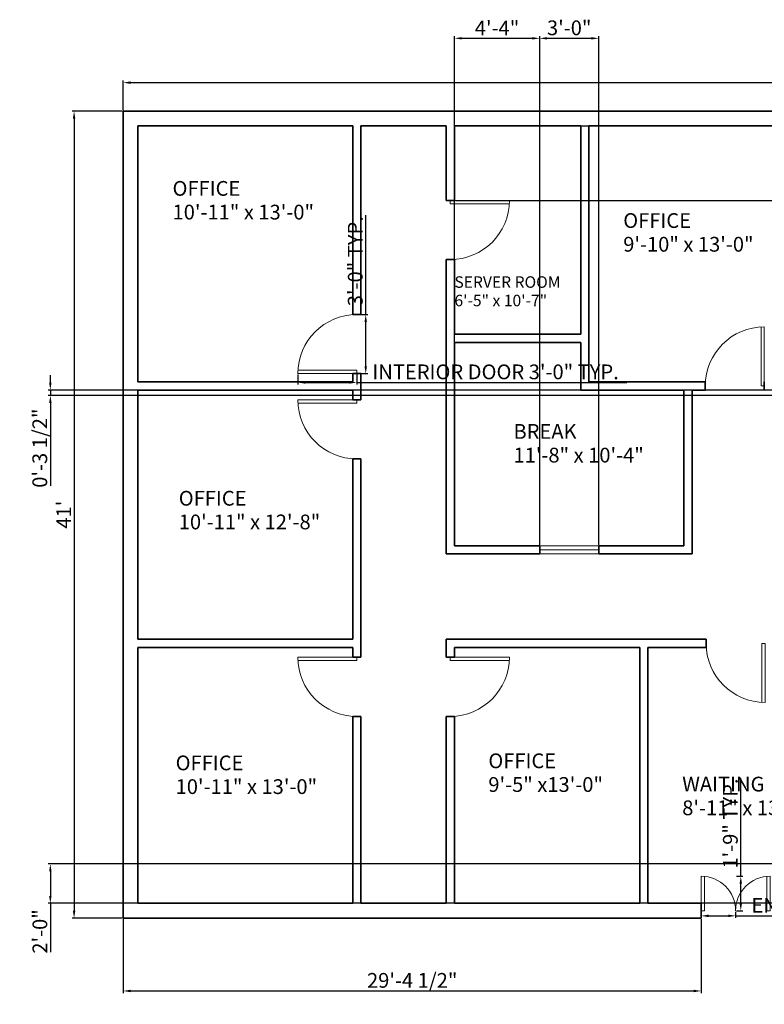
# Model space of a CAD drawing. Units: inches. Extents: x 2070 to 3026, y 1437 to 2044.
# Tile 1 of 2: x 2070 to 2524, y 1437 to 2037. Entities that reach past the tile are written whole.
import ezdxf

# ---------------------------------------------------------------- set-up
doc = ezdxf.new("R2010")
doc.units = ezdxf.units.IN
doc.layers.add('A-ANNO-DIMS', color=11, linetype='Continuous', lineweight=18, true_color=0xf27172)
doc.layers.add('A-GLAZ', color=11, linetype='Continuous', lineweight=18, true_color=0xf27172)
for name, color, linetype, lineweight in [('A-AREA-IDEN', 7, 'Continuous', 18), ('A-DOOR', 4, 'Continuous', 18), ('A-WALL', 7, 'Continuous', 35)]:
    doc.layers.add(name, color=color, linetype=linetype, lineweight=lineweight)
doc.styles.get("Standard").update_dxf_attribs({"font": 'arial.ttf'})
doc.dimstyles.new('ISO-25', dxfattribs={"dimtxt": 9, "dimasz": 4.5, "dimexe": 1.25, "dimexo": 0.625, "dimtad": 1, "dimdec": 0, "dimlunit": 3, "dimtxsty": 'Standard', "dimcen": 2.5, "dimadec": 0, "dimazin": 0, "dimtfac": 1, "dimtdec": 0, "dimtmove": 0, "dimatfit": 3, "dimfxl": 1, "dimarcsym": 0})

# ---------------------------------------------------------------- blocks, each defined once
blk = doc.blocks.new('*D3')
at = {"layer": 'A-ANNO-DIMS', "color": 0, "lineweight": -2, "transparency": 16777216}
for p, q in [((2133.31, 1981.8), (2133.31, 1999.85)), ((2973.31, 1981.8), (2973.31, 1999.85)), ((2137.81, 1998.6), (2968.81, 1998.6))]:
    blk.add_line(p, q, dxfattribs=at)
at = {"layer": 'A-ANNO-DIMS', "color": 0, "transparency": 16777216}
for points in [[(2137.81, 1999.35), (2137.81, 1997.85), (2133.31, 1998.6)], [(2968.81, 1999.35), (2968.81, 1997.85), (2973.31, 1998.6)]]:
    blk.add_solid(points, dxfattribs=at)
at = {"layer": 'Defpoints', "color": 0, "transparency": 16777216}
for p in [(2973.31, 1998.6), (2133.31, 1981.17), (2973.31, 1981.17)]:
    blk.add_point(p, dxfattribs=at)
at = {"layer": 'A-ANNO-DIMS', "color": 0, "transparency": 16777216, "insert": (2553.31, 2003.82), "char_height": 9, "attachment_point": 5}
blk.add_mtext("70'", dxfattribs=at)
blk = doc.blocks.new('*D4')
at = {"layer": 'A-ANNO-DIMS', "color": 0, "lineweight": -2, "transparency": 16777216}
for p, q in [((2132.69, 1981.17), (2102.08, 1981.17)), ((2103.33, 1976.67), (2103.33, 1493.67)), ((2132.69, 1489.17), (2102.08, 1489.17))]:
    blk.add_line(p, q, dxfattribs=at)
at = {"layer": 'A-ANNO-DIMS', "color": 0, "transparency": 16777216}
for points in [[(2102.58, 1976.67), (2104.08, 1976.67), (2103.33, 1981.17)], [(2102.58, 1493.67), (2104.08, 1493.67), (2103.33, 1489.17)]]:
    blk.add_solid(points, dxfattribs=at)
at = {"layer": 'Defpoints', "color": 0, "transparency": 16777216}
for p in [(2133.31, 1981.17), (2103.33, 1489.17), (2133.31, 1489.17)]:
    blk.add_point(p, dxfattribs=at)
at = {"layer": 'A-ANNO-DIMS', "color": 0, "transparency": 16777216, "insert": (2098.19, 1735.17), "char_height": 9, "attachment_point": 5, "rotation": 90}
blk.add_mtext("41'", dxfattribs=at)
blk = doc.blocks.new('DOOR-SWING-36IN')
for p, q in [((0, 2), (36, 2)), ((36, 0), (36, 2)), ((0, 0), (36, 0))]:
    blk.add_line(p, q)
blk.add_arc((36, 0), 36, 90, 180)
blk = doc.blocks.new('DOOR-ENTRY-LEAF-21IN')
for p, q in [((0, 21), (0, 0)), ((2, 21), (2, 0)), ((0, 0), (2, 0))]:
    blk.add_line(p, q)
blk.add_arc((0, 0), 21, 0, 90)
blk = doc.blocks.new('*D7')
at = {"layer": 'A-ANNO-DIMS', "color": 0, "lineweight": -2, "transparency": 16777216}
for p, q in [((2239.81, 1820.55), (2239.81, 1814.52)), ((2275.81, 1820.55), (2275.81, 1814.52)), ((2244.31, 1815.77), (2271.31, 1815.77)), ((2275.81, 1815.77), (2440.55, 1815.77))]:
    blk.add_line(p, q, dxfattribs=at)
at = {"layer": 'A-ANNO-DIMS', "color": 0, "transparency": 16777216}
for points in [[(2244.31, 1816.52), (2244.31, 1815.02), (2239.81, 1815.77)], [(2271.31, 1816.52), (2271.31, 1815.02), (2275.81, 1815.77)]]:
    blk.add_solid(points, dxfattribs=at)
at = {"layer": 'Defpoints', "color": 0, "transparency": 16777216}
for p in [(2239.81, 1821.17), (2275.81, 1821.17), (2275.81, 1815.77)]:
    blk.add_point(p, dxfattribs=at)
at = {"layer": 'A-ANNO-DIMS', "color": 0, "transparency": 16777216, "insert": (2360.43, 1821.06), "char_height": 9, "attachment_point": 5}
blk.add_mtext('INTERIOR DOOR 3\'-0" TYP.', dxfattribs=at)
blk = doc.blocks.new('*D8')
at = {"layer": 'A-ANNO-DIMS', "color": 0, "lineweight": -2, "transparency": 16777216}
for p, q in [((2281.21, 1857.17), (2281.21, 1917.78)), ((2276.44, 1857.17), (2282.46, 1857.17)), ((2281.21, 1825.67), (2281.21, 1852.67)), ((2276.44, 1821.17), (2282.46, 1821.17))]:
    blk.add_line(p, q, dxfattribs=at)
at = {"layer": 'A-ANNO-DIMS', "color": 0, "transparency": 16777216}
for points in [[(2280.46, 1852.67), (2281.96, 1852.67), (2281.21, 1857.17)], [(2280.46, 1825.67), (2281.96, 1825.67), (2281.21, 1821.17)]]:
    blk.add_solid(points, dxfattribs=at)
at = {"layer": 'Defpoints', "color": 0, "transparency": 16777216}
for p in [(2275.81, 1857.17), (2281.21, 1857.17), (2275.81, 1821.17)]:
    blk.add_point(p, dxfattribs=at)
at = {"layer": 'A-ANNO-DIMS', "color": 0, "transparency": 16777216, "insert": (2275.99, 1889.72), "char_height": 9, "attachment_point": 5, "rotation": 90}
blk.add_mtext('3\'-0" TYP.', dxfattribs=at)
blk = doc.blocks.new('*D9')
at = {"layer": 'A-ANNO-DIMS', "color": 0, "lineweight": -2, "transparency": 16777216}
for p, q in [((2485.81, 1493.05), (2485.81, 1489.27)), ((2490.31, 1490.52), (2502.31, 1490.52)), ((2506.81, 1493.05), (2506.81, 1489.27)), ((2506.81, 1490.52), (2647.99, 1490.52))]:
    blk.add_line(p, q, dxfattribs=at)
at = {"layer": 'A-ANNO-DIMS', "color": 0, "transparency": 16777216}
for points in [[(2490.31, 1491.27), (2490.31, 1489.77), (2485.81, 1490.52)], [(2502.31, 1491.27), (2502.31, 1489.77), (2506.81, 1490.52)]]:
    blk.add_solid(points, dxfattribs=at)
at = {"layer": 'Defpoints', "color": 0, "transparency": 16777216}
for p in [(2485.81, 1493.67), (2506.81, 1493.67), (2506.81, 1490.52)]:
    blk.add_point(p, dxfattribs=at)
at = {"layer": 'A-ANNO-DIMS', "color": 0, "transparency": 16777216, "insert": (2579.65, 1495.74), "char_height": 9, "attachment_point": 5}
blk.add_mtext('ENTRY LEAF 1\'-9" TYP.', dxfattribs=at)
blk = doc.blocks.new('*D10')
at = {"layer": 'A-ANNO-DIMS', "color": 0, "lineweight": -2, "transparency": 16777216}
for p, q in [((2509.96, 1514.67), (2509.96, 1574.44)), ((2507.44, 1514.67), (2511.21, 1514.67)), ((2509.96, 1498.17), (2509.96, 1510.17)), ((2507.44, 1493.67), (2511.21, 1493.67))]:
    blk.add_line(p, q, dxfattribs=at)
at = {"layer": 'A-ANNO-DIMS', "color": 0, "transparency": 16777216}
for points in [[(2509.21, 1510.17), (2510.71, 1510.17), (2509.96, 1514.67)], [(2509.21, 1498.17), (2510.71, 1498.17), (2509.96, 1493.67)]]:
    blk.add_solid(points, dxfattribs=at)
at = {"layer": 'Defpoints', "color": 0, "transparency": 16777216}
for p in [(2506.81, 1514.67), (2509.96, 1514.67), (2506.81, 1493.67)]:
    blk.add_point(p, dxfattribs=at)
at = {"layer": 'A-ANNO-DIMS', "color": 0, "transparency": 16777216, "insert": (2504.74, 1546.8), "char_height": 9, "attachment_point": 5, "rotation": 90}
blk.add_mtext('1\'-9" TYP.', dxfattribs=at)
blk = doc.blocks.new('*D17')
at = {"layer": 'A-ANNO-DIMS', "color": 0, "lineweight": -2, "transparency": 16777216}
for p, q in [((2335.311043, 1716.797797), (2335.311043, 2026.872797)), ((2339.811043, 2025.622797), (2382.811043, 2025.622797)), ((2387.311043, 1716.797797), (2387.311043, 2026.872797))]:
    blk.add_line(p, q, dxfattribs=at)
at = {"layer": 'A-ANNO-DIMS', "color": 0, "transparency": 16777216}
for points in [[(2339.811043, 2026.372797), (2339.811043, 2024.872797), (2335.311043, 2025.622797)], [(2382.811043, 2026.372797), (2382.811043, 2024.872797), (2387.311043, 2025.622797)]]:
    blk.add_solid(points, dxfattribs=at)
at = {"layer": 'Defpoints', "color": 0, "transparency": 16777216}
for p in [(2387.311043, 2025.622797), (2335.311043, 1716.172797), (2387.311043, 1716.172797)]:
    blk.add_point(p, dxfattribs=at)
at = {"layer": 'A-ANNO-DIMS', "color": 0, "transparency": 16777216, "insert": (2361.311043, 2030.747797), "char_height": 9, "attachment_point": 5}
blk.add_mtext('4\'-4"', dxfattribs=at)
blk = doc.blocks.new('*D18')
at = {"layer": 'A-ANNO-DIMS', "color": 0, "lineweight": -2, "transparency": 16777216}
for p, q in [((2387.31, 1716.8), (2387.31, 2026.87)), ((2391.81, 2025.62), (2418.81, 2025.62)), ((2423.31, 1716.8), (2423.31, 2026.87))]:
    blk.add_line(p, q, dxfattribs=at)
at = {"layer": 'A-ANNO-DIMS', "color": 0, "transparency": 16777216}
for points in [[(2391.81, 2026.37), (2391.81, 2024.87), (2387.31, 2025.62)], [(2418.81, 2026.37), (2418.81, 2024.87), (2423.31, 2025.62)]]:
    blk.add_solid(points, dxfattribs=at)
at = {"layer": 'Defpoints', "color": 0, "transparency": 16777216}
for p in [(2423.31, 2025.62), (2387.31, 1716.17), (2423.31, 1716.17)]:
    blk.add_point(p, dxfattribs=at)
at = {"layer": 'A-ANNO-DIMS', "color": 0, "transparency": 16777216, "insert": (2405.31, 2030.85), "char_height": 9, "attachment_point": 5}
blk.add_mtext('3\'-0"', dxfattribs=at)
blk = doc.blocks.new('*D19')
at = {"layer": 'A-ANNO-DIMS', "color": 0, "lineweight": -2, "transparency": 16777216}
for p, q in [((2335.94, 1972.17), (3019.01, 1972.17)), ((3017.76, 1967.67), (3017.76, 1931.17)), ((2335.94, 1926.67), (3019.01, 1926.67)), ((3017.76, 1926.67), (3017.76, 1876.03))]:
    blk.add_line(p, q, dxfattribs=at)
at = {"layer": 'A-ANNO-DIMS', "color": 0, "transparency": 16777216}
for points in [[(3017.01, 1967.67), (3018.51, 1967.67), (3017.76, 1972.17)], [(3017.01, 1931.17), (3018.51, 1931.17), (3017.76, 1926.67)]]:
    blk.add_solid(points, dxfattribs=at)
at = {"layer": 'Defpoints', "color": 0, "transparency": 16777216}
for p in [(2335.31, 1972.17), (2335.31, 1926.67), (3017.76, 1926.67)]:
    blk.add_point(p, dxfattribs=at)
at = {"layer": 'A-ANNO-DIMS', "color": 0, "transparency": 16777216, "insert": (3012.48, 1899.1), "char_height": 9, "attachment_point": 5, "rotation": 90}
blk.add_mtext('3\'-9 1/2"', dxfattribs=at)
blk = doc.blocks.new('*D20')
at = {"layer": 'A-ANNO-DIMS', "color": 0, "lineweight": -2, "transparency": 16777216}
for p, q in [((2133.31, 1488.55), (2133.31, 1443.47)), ((2485.81, 1488.55), (2485.81, 1443.47)), ((2137.81, 1444.72), (2481.31, 1444.72))]:
    blk.add_line(p, q, dxfattribs=at)
at = {"layer": 'A-ANNO-DIMS', "color": 0, "transparency": 16777216}
for points in [[(2137.81, 1445.47), (2137.81, 1443.97), (2133.31, 1444.72)], [(2481.31, 1445.47), (2481.31, 1443.97), (2485.81, 1444.72)]]:
    blk.add_solid(points, dxfattribs=at)
at = {"layer": 'Defpoints', "color": 0, "transparency": 16777216}
for p in [(2133.31, 1489.17), (2485.81, 1489.17), (2485.81, 1444.72)]:
    blk.add_point(p, dxfattribs=at)
at = {"layer": 'A-ANNO-DIMS', "color": 0, "transparency": 16777216, "insert": (2309.56, 1450), "char_height": 9, "attachment_point": 5}
blk.add_mtext('29\'-4 1/2"', dxfattribs=at)
blk = doc.blocks.new('*D26')
at = {"layer": 'A-ANNO-DIMS', "color": 0, "lineweight": -2, "transparency": 16777216}
for p, q in [((2088.86, 1815.67), (2088.86, 1820.17)), ((2593.69, 1811.17), (2087.61, 1811.17)), ((2606.2, 1807.8), (2087.61, 1807.8)), ((2088.86, 1811.17), (2088.86, 1807.8)), ((2088.86, 1803.3), (2088.86, 1752.65))]:
    blk.add_line(p, q, dxfattribs=at)
at = {"layer": 'A-ANNO-DIMS', "color": 0, "transparency": 16777216}
for points in [[(2088.11, 1815.67), (2089.61, 1815.67), (2088.86, 1811.17)], [(2088.11, 1803.3), (2089.61, 1803.3), (2088.86, 1807.8)]]:
    blk.add_solid(points, dxfattribs=at)
at = {"layer": 'Defpoints', "color": 0, "transparency": 16777216}
for p in [(2088.86, 1807.8), (2594.31, 1811.17), (2606.83, 1807.8)]:
    blk.add_point(p, dxfattribs=at)
at = {"layer": 'A-ANNO-DIMS', "color": 0, "transparency": 16777216, "insert": (2083.58, 1775.72), "char_height": 9, "attachment_point": 5, "rotation": 90}
blk.add_mtext('0\'-3 1/2"', dxfattribs=at)
blk = doc.blocks.new('*D31')
at = {"layer": 'A-ANNO-DIMS', "color": 0, "lineweight": -2, "transparency": 16777216}
for p, q in [((2564.69, 1522.17), (2087.61, 1522.17)), ((2088.86, 1517.67), (2088.86, 1502.67)), ((2564.69, 1498.17), (2087.61, 1498.17)), ((2088.86, 1498.17), (2088.86, 1468.35))]:
    blk.add_line(p, q, dxfattribs=at)
at = {"layer": 'A-ANNO-DIMS', "color": 0, "transparency": 16777216}
for points in [[(2088.11, 1517.67), (2089.61, 1517.67), (2088.86, 1522.17)], [(2088.11, 1502.67), (2089.61, 1502.67), (2088.86, 1498.17)]]:
    blk.add_solid(points, dxfattribs=at)
at = {"layer": 'Defpoints', "color": 0, "transparency": 16777216}
for p in [(2565.31, 1522.17), (2088.86, 1498.17), (2565.31, 1498.17)]:
    blk.add_point(p, dxfattribs=at)
at = {"layer": 'A-ANNO-DIMS', "color": 0, "transparency": 16777216, "insert": (2083.64, 1481.01), "char_height": 9, "attachment_point": 5, "rotation": 90}
blk.add_mtext('2\'-0"', dxfattribs=at)

msp = doc.modelspace()

# ---------------------------------------------------------------- linework, layer by layer
at = {"layer": 'A-GLAZ'}
for p, q in [((2387.31, 1716.17), (2423.31, 1716.17)), ((2387.31, 1713.67), (2423.31, 1713.67)), ((2387.31, 1711.17), (2423.31, 1711.17))]:
    msp.add_line(p, q, dxfattribs=at)
at = {"layer": 'A-WALL'}
for p, q in [((2133.31, 1981.17), (2973.31, 1981.17)), ((2133.31, 1489.17), (2133.31, 1981.17)), ((2142.31, 1972.17), (2273.31, 1972.17)), ((2142.31, 1816.17), (2142.31, 1972.17)), ((2273.31, 1857.17), (2273.31, 1972.17)), ((2278.31, 1857.17), (2278.31, 1972.17)), ((2278.31, 1972.17), (2330.31, 1972.17)), ((2330.31, 1926.67), (2330.31, 1972.17)), ((2335.31, 1972.17), (2412.31, 1972.17)), ((2335.31, 1972.17), (2335.31, 1926.67)), ((2335.31, 1926.67), (2335.31, 1972.17)), ((2412.31, 1845.17), (2412.31, 1972.17)), ((2417.31, 1816.17), (2417.31, 1972.17)), ((2417.31, 1972.17), (2530.31, 1972.17)), ((2335.31, 1926.67), (2330.31, 1926.67)), ((2330.31, 1711.17), (2330.31, 1890.67)), ((2335.31, 1890.67), (2330.31, 1890.67)), ((2335.31, 1845.17), (2335.31, 1890.67)), ((2335.31, 1890.67), (2335.31, 1845.17)), ((2273.31, 1857.17), (2278.31, 1857.17)), ((2335.31, 1845.17), (2412.31, 1845.17)), ((2335.31, 1840.17), (2412.31, 1840.17)), ((2335.31, 1716.17), (2335.31, 1840.17)), ((2412.31, 1811.17), (2412.31, 1840.17)), ((2273.31, 1821.17), (2278.31, 1821.17)), ((2273.31, 1816.17), (2273.31, 1821.17)), ((2278.31, 1805.17), (2278.31, 1821.17)), ((2142.31, 1816.17), (2273.31, 1816.17)), ((2417.31, 1816.17), (2488.31, 1816.17)), ((2488.31, 1811.17), (2488.31, 1816.17)), ((2524.31, 1811.17), (2524.31, 1816.17)), ((2142.31, 1811.17), (2273.31, 1811.17)), ((2142.31, 1659.17), (2142.31, 1811.17)), ((2273.31, 1805.17), (2273.31, 1811.17)), ((2412.31, 1811.17), (2475.31, 1811.17)), ((2475.31, 1716.17), (2475.31, 1811.17)), ((2480.31, 1711.17), (2480.31, 1811.17)), ((2480.31, 1811.17), (2488.31, 1811.17)), ((2273.31, 1805.17), (2278.31, 1805.17)), ((2273.31, 1769.17), (2278.31, 1769.17)), ((2273.31, 1659.17), (2273.31, 1769.17)), ((2278.31, 1648.17), (2278.31, 1769.17)), ((2330.31, 1711.17), (2387.31, 1711.17)), ((2335.31, 1716.17), (2387.31, 1716.17)), ((2387.31, 1711.17), (2387.31, 1716.17)), ((2423.31, 1716.17), (2475.31, 1716.17)), ((2423.31, 1711.17), (2423.31, 1716.17)), ((2423.31, 1711.17), (2480.31, 1711.17)), ((2273.31, 1659.17), (2142.31, 1659.17)), ((2330.31, 1648.17), (2330.31, 1659.17)), ((2488.81, 1659.17), (2330.31, 1659.17)), ((2488.81, 1654.17), (2488.81, 1659.17)), ((2142.31, 1498.17), (2142.31, 1654.17)), ((2273.31, 1654.17), (2142.31, 1654.17)), ((2273.31, 1648.17), (2273.31, 1654.17)), ((2335.31, 1648.17), (2335.31, 1654.17)), ((2448.31, 1654.17), (2335.31, 1654.17)), ((2448.31, 1498.17), (2448.31, 1654.17)), ((2453.31, 1498.17), (2453.31, 1654.17)), ((2453.31, 1654.17), (2488.81, 1654.17)), ((2488.81, 1654.17), (2453.31, 1654.17)), ((2278.31, 1648.17), (2273.31, 1648.17)), ((2335.31, 1648.17), (2330.31, 1648.17)), ((2273.31, 1498.17), (2273.31, 1612.17)), ((2278.31, 1612.17), (2273.31, 1612.17)), ((2278.31, 1498.17), (2278.31, 1612.17)), ((2330.31, 1498.17), (2330.31, 1612.17)), ((2335.31, 1612.17), (2330.31, 1612.17)), ((2335.31, 1498.17), (2335.31, 1612.17)), ((2273.31, 1498.17), (2142.31, 1498.17)), ((2330.31, 1498.17), (2278.31, 1498.17)), ((2448.31, 1498.17), (2335.31, 1498.17)), ((2485.81, 1498.17), (2453.31, 1498.17)), ((2485.81, 1498.17), (2453.31, 1498.17)), ((2485.81, 1498.17), (2485.81, 1489.17)), ((2485.81, 1489.17), (2133.31, 1489.17))]:
    msp.add_line(p, q, dxfattribs=at)

# ---------------------------------------------------------------- block references
at = {"layer": 'A-DOOR'}
for p, rotation in [((2368.81, 1926.67), 180), ((2524.81, 1620.67), 89.99999999999994), ((2368.81, 1648.17), 180)]:
    msp.add_blockref('DOOR-SWING-36IN', p, dxfattribs=dict(at, rotation=rotation))
for name, p in [('DOOR-SWING-36IN', (2239.81, 1821.17)), ('DOOR-ENTRY-LEAF-21IN', (2485.81, 1493.67))]:
    msp.add_blockref(name, p, dxfattribs=at)
at = {"layer": 'A-DOOR', "extrusion": (0, 0, -1), "zscale": -1}
for p, rotation in [((-2524.31, 1849.67), 270.0000000000001), ((-2239.81, 1805.17), 180), ((-2239.81, 1648.17), 180)]:
    msp.add_blockref('DOOR-SWING-36IN', p, dxfattribs=dict(at, rotation=rotation))
msp.add_blockref('DOOR-ENTRY-LEAF-21IN', (-2527.81, 1493.67), dxfattribs=at)

# ---------------------------------------------------------------- texts
at = {"layer": 'A-AREA-IDEN'}
for s, height, p in [('OFFICE', 9, (2163.38, 1929.6)), ('10\'-11" x 13\'-0"', 9, (2163.38, 1915.15)), ('OFFICE', 9, (2438.27, 1910)), ('9\'-10" x 13\'-0"', 9, (2438.27, 1895.54)), ('SERVER ROOM  ', 7, (2335.31, 1873.49)), ('6\'-5" x 10\'-7"', 7, (2335.31, 1862.24)), ('BREAK', 9, (2371.32, 1781.42)), ('11\'-8" x 10\'-4"', 9, (2371.32, 1766.96)), ('OFFICE', 9, (2167.17, 1740.66)), ('10\'-11" x 12\'-8"', 9, (2167.17, 1726.21)), ('OFFICE', 9, (2165.27, 1579.28)), ('OFFICE', 9, (2356, 1580.56)), ('10\'-11" x 13\'-0"', 9, (2165.27, 1564.82)), ('9\'-5" x13\'-0"', 9, (2356, 1566.1)), ('WAITING', 9, (2474.24, 1566.36)), ('8\'-11" x 13\'-0"', 9, (2474.24, 1551.9))]:
    msp.add_text(s, height=height, dxfattribs=at).set_placement(p)

# ---------------------------------------------------------------- dimensions: what is measured, and where the dimension line sits
at = {"layer": 'A-ANNO-DIMS'}
for base, p1, p2, override, picture, middle in [((2387.31, 2025.62), (2335.31, 1716.17), (2387.31, 1716.17), {"dimdec": 1, "dimlfac": 1, "dimrnd": 0, "dimzin": 1, "dimdsep": 46, "dimlunit": 4, "dimfrac": 2}, '*D17', (2361.31, 2030.75)), ((2423.31, 2025.62), (2387.31, 1716.17), (2423.31, 1716.17), {"dimdec": 1, "dimlfac": 1, "dimrnd": 0, "dimzin": 1, "dimdsep": 46, "dimlunit": 4, "dimfrac": 2}, '*D18', (2405.31, 2030.85)), ((2973.31, 1998.6), (2133.31, 1981.17), (2973.31, 1981.17), {"dimclrd": 0, "dimclre": 0, "dimclrt": 0}, '*D3', (2553.31, 2003.82)), ((2485.81, 1444.72), (2133.31, 1489.17), (2485.81, 1489.17), {"dimdec": 1, "dimlfac": 1, "dimrnd": 0, "dimzin": 1, "dimdsep": 46, "dimlunit": 4, "dimfrac": 2}, '*D20', (2309.56, 1450))]:
    dim = msp.add_linear_dim(base=base, p1=p1, p2=p2, dimstyle='ISO-25', override=override, dxfattribs=at)
    dim.commit()
    dim.dimension.update_dxf_attribs({"geometry": picture, "text_midpoint": middle})
for base, p1, p2, override, picture, middle in [((2103.33, 1489.17), (2133.31, 1981.17), (2133.31, 1489.17), {"dimclrd": 0, "dimclre": 0, "dimclrt": 0}, '*D4', (2098.19, 1735.17)), ((3017.76, 1926.67), (2335.31, 1972.17), (2335.31, 1926.67), {"dimdec": 1, "dimlfac": 1, "dimrnd": 0, "dimzin": 1, "dimdsep": 46, "dimlunit": 4, "dimfrac": 2}, '*D19', (3012.48, 1899.1)), ((2088.86, 1807.8), (2594.31, 1811.17), (2606.83, 1807.8), {"dimdec": 1, "dimlfac": 1, "dimrnd": 0, "dimzin": 1, "dimdsep": 46, "dimlunit": 4, "dimfrac": 2}, '*D26', (2083.58, 1775.72)), ((2088.86, 1498.17), (2565.31, 1522.17), (2565.31, 1498.17), {"dimdec": 1, "dimlfac": 1, "dimrnd": 0, "dimzin": 1, "dimdsep": 46, "dimlunit": 4, "dimfrac": 2}, '*D31', (2083.64, 1481.01))]:
    dim = msp.add_linear_dim(base=base, p1=p1, p2=p2, angle=90, dimstyle='ISO-25', override=override, dxfattribs=at)
    dim.commit()
    dim.dimension.update_dxf_attribs({"geometry": picture, "text_midpoint": middle})
for base, p1, p2, picture, middle in [((2281.21, 1857.17), (2275.81, 1821.17), (2275.81, 1857.17), '*D8', (2275.99, 1889.72)), ((2509.96, 1514.67), (2506.81, 1493.67), (2506.81, 1514.67), '*D10', (2504.74, 1546.8))]:
    dim = msp.add_linear_dim(base=base, p1=p1, p2=p2, angle=90, text='<> TYP.', dimstyle='ISO-25', override={"dimdec": 1, "dimlfac": 1, "dimrnd": 0, "dimzin": 1, "dimdsep": 46, "dimlunit": 4, "dimfrac": 2}, dxfattribs=at)
    dim.commit()
    dim.dimension.update_dxf_attribs({"geometry": picture, "text_midpoint": middle})
for base, p1, p2, text, picture, middle in [((2275.81, 1815.77), (2239.81, 1821.17), (2275.81, 1821.17), 'INTERIOR DOOR <> TYP.', '*D7', (2360.43, 1821.06)), ((2506.81, 1490.52), (2485.81, 1493.67), (2506.81, 1493.67), 'ENTRY LEAF <> TYP.', '*D9', (2579.65, 1495.74))]:
    dim = msp.add_linear_dim(base=base, p1=p1, p2=p2, text=text, dimstyle='ISO-25', override={"dimdec": 1, "dimlfac": 1, "dimrnd": 0, "dimzin": 1, "dimdsep": 46, "dimlunit": 4, "dimfrac": 2}, dxfattribs=at)
    dim.commit()
    dim.dimension.update_dxf_attribs({"geometry": picture, "text_midpoint": middle})

doc.saveas('drawing.dxf')
